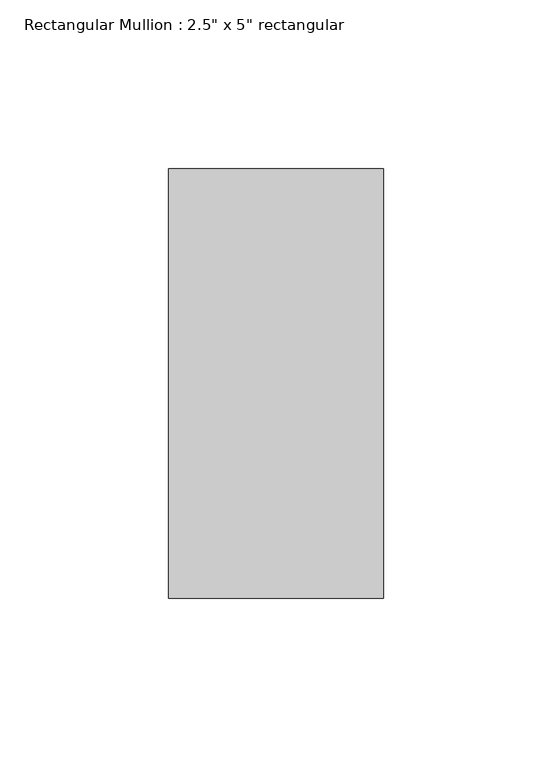
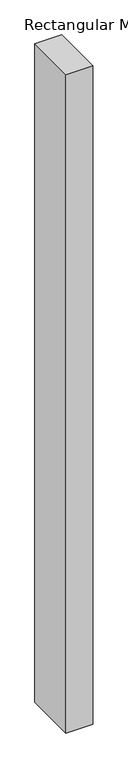
"""IFC4 building model written with IfcOpenShell, lengths in millimetres: member geometry."""

from ifc_helpers import new_model, si_unit, frame, origin, place, context, project, spatial, polyline, outline, extrude, source, transform, mapped, element, save


def member_25a9efec(model_context):
    return source(origin(), model_context, "Body", "SweptSolid", [
        extrude(outline(polyline([(31.75, 63.5), (31.75, -63.5), (-31.75, -63.5), (-31.75, 63.5), (31.75, 63.5)])), frame((0.0, 0.0, -1644.3056511), z_axis=(0.0, 0.0, 1.0), x_axis=(1.0, 0.0, 0.0)), (0.0, 0.0, 1.0), 1644.3056511),
    ])


if __name__ == "__main__":
    model = new_model("IFC4")
    model_context = context("Model", 3, world=origin())
    ifc_project = project(units=[si_unit("LENGTHUNIT", "METRE", prefix="MILLI")], contexts=[model_context])
    site = spatial("IfcSite", under=ifc_project)
    building = spatial("IfcBuilding", under=site)
    placement = place(None, origin())
    member_shape = member_25a9efec(model_context)
    element("IfcMember", 1, ObjectType="Rectangular Mullion : 2.5\" x 5\" rectangular", at=placement, inside=building, context=model_context, shape_type="MappedRepresentation", body=[
        mapped(member_shape, transform((0.0, 0.0, 0.0), x_axis=(1.0, 0.0, 0.0), y_axis=(0.0, 1.0, 0.0), z_axis=(0.0, 0.0, 1.0))),
    ])
    save(model, "model.ifc")

# Revit data of these elements
# Type "Rectangular Mullion : 2.5\" x 5\" rectangular"
#   built-in parameter 1007304 = 0.416667 (stored number, unit not read)
#   built-in parameter 1007301 = 0.104167 (stored number, unit not read)
#   built-in parameter 1007300 = 0.104167 (stored number, unit not read)
# Element 1 (IfcMember, "Rectangular Mullion : 2.5\" x 5\" rectangular")
#   Materials on its faces: "Aluminum"
# Materials
#   "Aluminum": class "Metal", colour RGB 247 247 247, transparency 0, Description = "Aluminum 6061", Cost = 0
